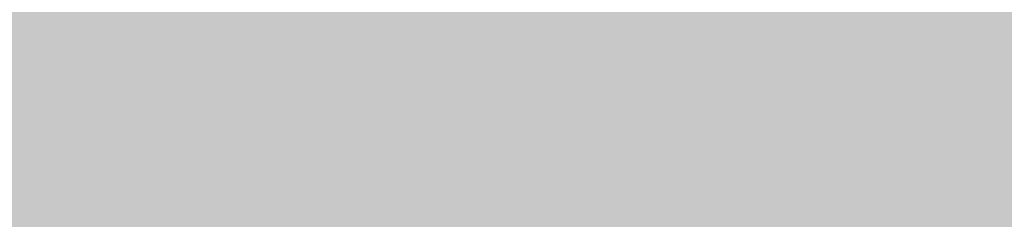
# Model space of a CAD drawing. Units: millimetres. Extents: x 0 to 2267, y 0 to 1823.
# Tile 78 of 256: x 1600.369 to 1605.705, y 1226.115 to 1227.196. Entities that reach past the tile are written whole.
import ezdxf

# ---------------------------------------------------------------- set-up
doc = ezdxf.new("R2010")
doc.units = ezdxf.units.MM
doc.header["$MEASUREMENT"] = 0
doc.layers.add('M-HATC', color=252, linetype='Continuous', lineweight=18)

msp = doc.modelspace()

# ---------------------------------------------------------------- hatches: boundary and pattern name
at = {"layer": 'M-HATC'}
h = msp.add_hatch(color=256, dxfattribs=at)
h.dxf.hatch_style = 1
h.paths.add_polyline_path([(2055.771, 1603.062), (1381.0868, 1603.062), (1381.0868, 1598.062), (2055.771, 1598.062)])
h.paths.add_polyline_path([(2055.771, 1598.062), (1381.0868, 1598.062), (1381.0868, 1593.062), (2055.771, 1593.062)])
h.paths.add_polyline_path([(2051.3074, 1536.7609), (1385.5504, 1536.7609), (1385.5504, 1526.7609), (1387.5504, 1526.7609), (1388.5366, 1525.0528), (1385.3319, 1521.2335), (1385.3319, 1521.2226), (2050.2542, 1522.7491), (2048.3212, 1525.0528), (2049.3074, 1526.7609), (2051.3074, 1526.7609)])
edge = h.paths.add_edge_path()
edge.add_arc((1847.5345, 1379.1492), 135, 222.603061, 222.890851, ccw=False)
edge.add_line((1748.1663, 1287.7656), (1683.0921, 1287.7656))
edge.add_arc((1583.7239, 1379.1492), 135, 317.109149, 317.396939, ccw=False)
edge.add_arc((1678.9686, 1290.6707), 5, 222.8909, 317.1091, ccw=False)
edge.add_arc((1774.2133, 1379.1492), 135, 222.603061, 222.890851, ccw=False)
edge.add_line((1674.8451, 1287.7656), (1609.7709, 1287.7656))
edge.add_arc((1510.4027, 1379.1492), 135, 317.109149, 317.396939, ccw=False)
edge.add_arc((1605.6474, 1290.6707), 5, 222.8909, 317.1091, ccw=False)
edge.add_arc((1700.8921, 1379.1492), 135, 222.603061, 222.890851, ccw=False)
edge.add_line((1601.5239, 1287.7656), (1536.4497, 1287.7656))
edge.add_arc((1437.0815, 1379.1492), 135, 317.109149, 317.396939, ccw=False)
edge.add_arc((1532.3262, 1290.6707), 5, 222.8909, 317.1091, ccw=False)
edge.add_arc((1627.5709, 1379.1492), 135, 222.603061, 222.890851, ccw=False)
edge.add_line((1528.2027, 1287.7656), (1505.9289, 1287.7656))
edge.add_spline(control_points=[(1505.9289, 1287.7656), (1504.2622, 1287.7656), (1504.2622, 1282.7656), (1505.9289, 1282.7656)], knot_values=[0, 0, 0, 0, 5, 5, 5, 5], degree=3, periodic=0)
edge.add_line((1505.9289, 1282.7656), (1930.9289, 1282.7656))
edge.add_spline(control_points=[(1930.9289, 1282.7656), (1932.5956, 1282.7656), (1932.5956, 1287.7656), (1930.9289, 1287.7656)], knot_values=[0, 0, 0, 0, 5, 5, 5, 5], degree=3, periodic=0)
edge.add_line((1930.9289, 1287.7656), (1903.0557, 1287.7656))
edge.add_arc((1803.6875, 1379.1492), 135, 317.109149, 317.396939, ccw=False)
edge.add_arc((1898.9322, 1290.6707), 5, 222.8909, 317.1091, ccw=False)
edge.add_arc((1994.1769, 1379.1492), 135, 222.603061, 222.890851, ccw=False)
edge.add_line((1894.8087, 1287.7656), (1829.7345, 1287.7656))
edge.add_arc((1730.3663, 1379.1492), 135, 317.109149, 317.396939, ccw=False)
edge.add_arc((1825.611, 1290.6707), 5, 222.8909, 317.1091, ccw=False)
edge.add_arc((1920.8557, 1379.1492), 135, 222.603061, 222.890851, ccw=False)
edge.add_line((1821.4875, 1287.7656), (1756.4133, 1287.7656))
edge.add_arc((1657.0451, 1379.1492), 135, 317.109149, 317.396939, ccw=False)
edge.add_arc((1752.2898, 1290.6707), 5, 222.8909, 317.1091, ccw=False)
edge = h.paths.add_edge_path()
edge.add_spline(control_points=[(1843.4289, 1227.2475), (1845.0956, 1227.2475), (1845.0956, 1232.2475), (1843.4289, 1232.2475)], knot_values=[0, 0, 0, 0, 5, 5, 5, 5], degree=3, periodic=0)
edge.add_line((1843.4289, 1232.2475), (1593.4289, 1232.2475))
edge.add_spline(control_points=[(1593.4289, 1232.2475), (1591.7622, 1232.2475), (1591.7622, 1227.2475), (1593.4289, 1227.2475)], knot_values=[0, 0, 0, 0, 5, 5, 5, 5], degree=3, periodic=0)
edge.add_line((1593.4289, 1227.2475), (1843.4289, 1227.2475))
h.paths.add_polyline_path([(1905.9289, 1127.4171), (1530.9289, 1127.4171, 0.414214), (1520.9289, 1117.4171), (1530.9289, 1117.4171), (1915.9289, 1117.4171, 0.414214)])
edge = h.paths.add_edge_path()
edge.add_arc((1397.0858, 1498.4078), 12.7299, 90.78215, 190.87871, ccw=False)
edge.add_line((1396.912, 1511.1365), (1428.0097, 1511.3488))
edge.add_line((1428.0097, 1511.3488), (1433.0097, 1511.3488))
edge.add_line((1433.0097, 1511.3488), (1434.439, 1511.3488))
edge.add_arc((1419.474, 1498.0804), 20, 41.561, 74.08211)
edge.add_line((1424.9592, 1517.3135), (1399.9351, 1517.2561))
edge.add_spline(control_points=[(1399.9307, 1517.2561), (1399.884, 1517.2131), (1399.8328, 1517.1689), (1399.7774, 1517.1236)], knot_values=[11.567499, 11.567499, 11.567499, 11.567499, 11.814249, 11.814249, 11.814249, 11.814249], degree=3, periodic=0)
edge.add_spline(control_points=[(1399.6328, 1517.0099), (1399.5831, 1516.9721), (1399.5307, 1516.9338), (1399.4759, 1516.8947)], knot_values=[11.167718, 11.167718, 11.167718, 11.167718, 11.365188, 11.365188, 11.365188, 11.365188], degree=3, periodic=0)
edge.add_spline(control_points=[(1399.3398, 1516.8001), (1399.1514, 1516.6719), (1398.9384, 1516.5377), (1398.704, 1516.3994)], knot_values=[10.376405, 10.376405, 10.376405, 10.376405, 11.00994, 11.00994, 11.00994, 11.00994], degree=3, periodic=0)
edge.add_spline(control_points=[(1398.6572, 1516.3719), (1398.5789, 1516.326), (1398.4983, 1516.2797), (1398.4155, 1516.2331)], knot_values=[10.125175, 10.125175, 10.125175, 10.125175, 10.334406, 10.334406, 10.334406, 10.334406], degree=3, periodic=0)
edge.add_spline(control_points=[(1398.2642, 1516.1487), (1398.196, 1516.1111), (1398.1263, 1516.0732), (1398.0555, 1516.0351)], knot_values=[9.832246, 9.832246, 9.832246, 9.832246, 9.999658, 9.999658, 9.999658, 9.999658], degree=3, periodic=0)
edge.add_spline(control_points=[(1397.9987, 1516.0048), (1397.7312, 1515.8621), (1397.446, 1515.7171), (1397.1466, 1515.5714)], knot_values=[9.161808, 9.161808, 9.161808, 9.161808, 9.787769, 9.787769, 9.787769, 9.787769], degree=3, periodic=0)
edge.add_spline(control_points=[(1397.1466, 1515.5714), (1396.8418, 1515.423), (1396.5222, 1515.274), (1396.1914, 1515.1262)], knot_values=[8.524455, 8.524455, 8.524455, 8.524455, 9.161808, 9.161808, 9.161808, 9.161808], degree=3, periodic=0)
edge.add_spline(control_points=[(1396.0777, 1515.0756), (1395.9854, 1515.0348), (1395.8922, 1514.994), (1395.7983, 1514.9534)], knot_values=[8.275193, 8.275193, 8.275193, 8.275193, 8.451726, 8.451726, 8.451726, 8.451726], degree=3, periodic=0)
edge.add_spline(control_points=[(1395.6018, 1514.8691), (1395.4997, 1514.8257), (1395.3968, 1514.7824), (1395.2932, 1514.7394)], knot_values=[7.962917, 7.962917, 7.962917, 7.962917, 8.152764, 8.152764, 8.152764, 8.152764], degree=3, periodic=0)
edge.add_spline(control_points=[(1395.2116, 1514.7057), (1394.8278, 1514.5475), (1394.4345, 1514.3929), (1394.0364, 1514.2442)], knot_values=[7.21254, 7.21254, 7.21254, 7.21254, 7.913148, 7.913148, 7.913148, 7.913148], degree=3, periodic=0)
edge.add_spline(control_points=[(1394.0364, 1514.2442), (1393.7076, 1514.1214), (1393.3754, 1514.0027), (1393.0427, 1513.8895)], knot_values=[6.633733, 6.633733, 6.633733, 6.633733, 7.21254, 7.21254, 7.21254, 7.21254], degree=3, periodic=0)
edge.add_spline(control_points=[(1392.8214, 1513.815), (1392.7198, 1513.7812), (1392.6181, 1513.7479), (1392.5166, 1513.7152)], knot_values=[6.328796, 6.328796, 6.328796, 6.328796, 6.505493, 6.505493, 6.505493, 6.505493], degree=3, periodic=0)
edge.add_spline(control_points=[(1392.5166, 1513.7152), (1392.3187, 1513.6515), (1392.1212, 1513.59), (1391.9244, 1513.531)], knot_values=[5.984605, 5.984605, 5.984605, 5.984605, 6.328796, 6.328796, 6.328796, 6.328796], degree=3, periodic=0)
edge.add_spline(control_points=[(1391.7915, 1513.4915), (1391.3122, 1513.3501), (1390.8384, 1513.2239), (1390.3784, 1513.1171)], knot_values=[5.066697, 5.066697, 5.066697, 5.066697, 5.907055, 5.907055, 5.907055, 5.907055], degree=3, periodic=0)
edge.add_spline(control_points=[(1390.3784, 1513.1171), (1390.1797, 1513.071), (1389.9836, 1513.0284), (1389.7907, 1512.9899)], knot_values=[4.70367, 4.70367, 4.70367, 4.70367, 5.066695, 5.066695, 5.066695, 5.066695], degree=3, periodic=0)
edge.add_spline(control_points=[(1389.422, 1512.9204), (1389.2459, 1512.8892), (1389.0729, 1512.8617), (1388.9036, 1512.8381)], knot_values=[4.130571, 4.130571, 4.130571, 4.130571, 4.469816, 4.469816, 4.469816, 4.469816], degree=3, periodic=0)
edge.add_spline(control_points=[(1388.9036, 1512.8381), (1388.591, 1512.7946), (1388.2911, 1512.7644), (1388.0071, 1512.7494)], knot_values=[3.504031, 3.504031, 3.504031, 3.504031, 4.130571, 4.130571, 4.130571, 4.130571], degree=3, periodic=0)
edge.add_spline(control_points=[(1387.9356, 1512.7459), (1387.8538, 1512.7423), (1387.7733, 1512.74), (1387.6944, 1512.739)], knot_values=[3.268866, 3.268866, 3.268866, 3.268866, 3.451164, 3.451164, 3.451164, 3.451164], degree=3, periodic=0)
edge.add_spline(control_points=[(1387.3351, 1512.7443), (1387.2076, 1512.7499), (1387.0847, 1512.7597), (1386.967, 1512.7739)], knot_values=[2.670686, 2.670686, 2.670686, 2.670686, 2.984, 2.984, 2.984, 2.984], degree=3, periodic=0)
edge.add_spline(control_points=[(1386.8327, 1512.7922), (1386.8209, 1512.7941), (1386.8092, 1512.7959), (1386.7975, 1512.7979)], knot_values=[2.516981, 2.516981, 2.516981, 2.516981, 2.549528, 2.549528, 2.549528, 2.549528], degree=3, periodic=0)
edge.add_spline(control_points=[(1386.4526, 1512.8735), (1386.4257, 1512.881), (1386.3993, 1512.889), (1386.3733, 1512.8972)], knot_values=[2.095869, 2.095869, 2.095869, 2.095869, 2.17941, 2.17941, 2.17941, 2.17941], degree=3, periodic=0)
edge.add_spline(control_points=[(1386.0691, 1513.0189), (1386.0634, 1513.0217), (1386.0577, 1513.0246), (1386.052, 1513.0275)], knot_values=[1.72453, 1.72453, 1.72453, 1.72453, 1.745933, 1.745933, 1.745933, 1.745933], degree=3, periodic=0)
edge.add_arc((1399.474, 1498.0804), 20, 131.82432, 180)
edge.add_arc((1630.3336, 1505.5484), 250.9708, 181.705176, 236.427975)
edge.add_arc((1605.3399, 1483.3044), 218.7822, 238.660829, 243.34961)
edge.add_arc((1647.0911, 1510.3592), 262.8986, 183.129836, 237.853442, ccw=False)
h.paths.add_polyline_path([(1406.5369, 1391.9644, 0.149382), (1491.5506, 1296.4418, -0.129517)], flags=17)
edge = h.paths.add_edge_path()
edge.add_arc((2037.3838, 1498.0804), 20, 0, 48.26587)
edge.add_spline(control_points=[(2050.6973, 1513.0052), (2050.6512, 1512.9847), (2050.6034, 1512.9655), (2050.5539, 1512.9477)], knot_values=[1.835652, 1.835652, 1.835652, 1.835652, 2.000781, 2.000781, 2.000781, 2.000781], degree=3, periodic=0)
edge.add_spline(control_points=[(2050.4616, 1512.9166), (2050.479, 1512.9221), (2050.4963, 1512.9277), (2050.5133, 1512.9335)], knot_values=[2.045477, 2.045477, 2.045477, 2.045477, 2.101389, 2.101389, 2.101389, 2.101389], degree=3, periodic=0)
edge.add_spline(control_points=[(2050.129, 1512.8342), (2050.1984, 1512.8473), (2050.2657, 1512.8623), (2050.3308, 1512.8792)], knot_values=[2.237629, 2.237629, 2.237629, 2.237629, 2.435841, 2.435841, 2.435841, 2.435841], degree=3, periodic=0)
edge.add_spline(control_points=[(2050.0946, 1512.8278), (2050.1061, 1512.8299), (2050.1176, 1512.832), (2050.129, 1512.8342)], knot_values=[2.435841, 2.435841, 2.435841, 2.435841, 2.468321, 2.468321, 2.468321, 2.468321], degree=3, periodic=0)
edge.add_spline(control_points=[(2049.7843, 1512.7851), (2049.8552, 1512.7922), (2049.9243, 1512.8008), (2049.9917, 1512.8109)], knot_values=[2.563852, 2.563852, 2.563852, 2.563852, 2.748541, 2.748541, 2.748541, 2.748541], degree=3, periodic=0)
edge.add_spline(control_points=[(2049.4052, 1512.7617), (2049.5364, 1512.7653), (2049.6629, 1512.773), (2049.7843, 1512.7851)], knot_values=[2.748541, 2.748541, 2.748541, 2.748541, 3.064882, 3.064882, 3.064882, 3.064882], degree=3, periodic=0)
edge.add_spline(control_points=[(2049.1698, 1512.7597), (2049.2336, 1512.7591), (2049.2965, 1512.7594), (2049.3584, 1512.7606)], knot_values=[3.102309, 3.102309, 3.102309, 3.102309, 3.2503, 3.2503, 3.2503, 3.2503], degree=3, periodic=0)
edge.add_spline(control_points=[(2048.8573, 1512.7691), (2048.9638, 1512.7638), (2049.068, 1512.7606), (2049.1698, 1512.7597)], knot_values=[3.2503, 3.2503, 3.2503, 3.2503, 3.486069, 3.486069, 3.486069, 3.486069], degree=3, periodic=0)
edge.add_spline(control_points=[(2048.6924, 1512.7789), (2048.3729, 1512.8009), (2048.0345, 1512.8411), (2047.6817, 1512.897)], knot_values=[3.606429, 3.606429, 3.606429, 3.606429, 4.2989, 4.2989, 4.2989, 4.2989], degree=3, periodic=0)
edge.add_spline(control_points=[(2047.6817, 1512.897), (2047.5458, 1512.9185), (2047.4077, 1512.9424), (2047.2678, 1512.9685)], knot_values=[4.2989, 4.2989, 4.2989, 4.2989, 4.565769, 4.565769, 4.565769, 4.565769], degree=3, periodic=0)
edge.add_spline(control_points=[(2047.2678, 1512.9685), (2047.1449, 1512.9914), (2047.0207, 1513.016), (2046.8951, 1513.0422)], knot_values=[4.565769, 4.565769, 4.565769, 4.565769, 4.799971, 4.799971, 4.799971, 4.799971], degree=3, periodic=0)
edge.add_spline(control_points=[(2046.8951, 1513.0422), (2046.5286, 1513.1188), (2046.1513, 1513.209), (2045.7676, 1513.3107)], knot_values=[4.799971, 4.799971, 4.799971, 4.799971, 5.483718, 5.483718, 5.483718, 5.483718], degree=3, periodic=0)
edge.add_spline(control_points=[(2045.7676, 1513.3107), (2045.3724, 1513.4154), (2044.9704, 1513.5322), (2044.5662, 1513.6588)], knot_values=[5.483718, 5.483718, 5.483718, 5.483718, 6.187866, 6.187866, 6.187866, 6.187866], degree=3, periodic=0)
edge.add_spline(control_points=[(2044.5662, 1513.6588), (2044.4149, 1513.7061), (2044.2633, 1513.7549), (2044.1116, 1513.8048)], knot_values=[6.187866, 6.187866, 6.187866, 6.187866, 6.451551, 6.451551, 6.451551, 6.451551], degree=3, periodic=0)
edge.add_spline(control_points=[(2044.1116, 1513.8048), (2043.9967, 1513.8427), (2043.8817, 1513.8813), (2043.7668, 1513.9205)], knot_values=[6.451551, 6.451551, 6.451551, 6.451551, 6.651434, 6.651434, 6.651434, 6.651434], degree=3, periodic=0)
edge.add_spline(control_points=[(2043.7668, 1513.9205), (2043.3716, 1514.0554), (2042.9774, 1514.1979), (2042.5886, 1514.3458)], knot_values=[6.651434, 6.651434, 6.651434, 6.651434, 7.338879, 7.338879, 7.338879, 7.338879], degree=3, periodic=0)
edge.add_spline(control_points=[(2042.5886, 1514.3458), (2042.1643, 1514.5071), (2041.7465, 1514.6749), (2041.3409, 1514.846)], knot_values=[7.338879, 7.338879, 7.338879, 7.338879, 8.089209, 8.089209, 8.089209, 8.089209], degree=3, periodic=0)
edge.add_spline(control_points=[(2041.3409, 1514.846), (2041.1028, 1514.9465), (2040.869, 1515.0481), (2040.6405, 1515.1502)], knot_values=[8.089209, 8.089209, 8.089209, 8.089209, 8.529587, 8.529587, 8.529587, 8.529587], degree=3, periodic=0)
edge.add_spline(control_points=[(2040.51, 1515.2089), (2040.0824, 1515.4022), (2039.6747, 1515.5971), (2039.295, 1515.7894)], knot_values=[8.613818, 8.613818, 8.613818, 8.613818, 9.44571, 9.44571, 9.44571, 9.44571], degree=3, periodic=0)
edge.add_spline(control_points=[(2039.295, 1515.7894), (2039.0618, 1515.9075), (2038.8391, 1516.0246), (2038.6288, 1516.1398)], knot_values=[9.44571, 9.44571, 9.44571, 9.44571, 9.956404, 9.956404, 9.956404, 9.956404], degree=3, periodic=0)
edge.add_spline(control_points=[(2038.6288, 1516.1398), (2038.5187, 1516.2001), (2038.4121, 1516.2598), (2038.309, 1516.3189)], knot_values=[9.956404, 9.956404, 9.956404, 9.956404, 10.223542, 10.223542, 10.223542, 10.223542], degree=3, periodic=0)
edge.add_spline(control_points=[(2038.309, 1516.3189), (2038.2138, 1516.3735), (2038.1216, 1516.4276), (2038.0328, 1516.481)], knot_values=[10.223542, 10.223542, 10.223542, 10.223542, 10.47051, 10.47051, 10.47051, 10.47051], degree=3, periodic=0)
edge.add_spline(control_points=[(2038.0328, 1516.481), (2037.7855, 1516.6296), (2037.5639, 1516.773), (2037.3722, 1516.909)], knot_values=[10.47051, 10.47051, 10.47051, 10.47051, 11.15767, 11.15767, 11.15767, 11.15767], degree=3, periodic=0)
edge.add_spline(control_points=[(2037.3722, 1516.909), (2037.2789, 1516.9752), (2037.1927, 1517.0396), (2037.1142, 1517.102)], knot_values=[11.15767, 11.15767, 11.15767, 11.15767, 11.49227, 11.49227, 11.49227, 11.49227], degree=3, periodic=0)
edge.add_spline(control_points=[(2036.8564, 1517.3259), (2036.9148, 1517.2692), (2036.9814, 1517.2103), (2037.0557, 1517.1492)], knot_values=[11.577341, 11.577341, 11.577341, 11.577341, 11.91035, 11.91035, 11.91035, 11.91035], degree=3, periodic=0)
edge.add_spline(control_points=[(2036.8074, 1517.3748), (2036.823, 1517.3587), (2036.8393, 1517.3424), (2036.8564, 1517.3259)], knot_values=[11.91035, 11.91035, 11.91035, 11.91035, 12.007402, 12.007402, 12.007402, 12.007402], degree=3, periodic=0)
edge.add_spline(control_points=[(2036.7017, 1517.494), (2036.7104, 1517.483), (2036.7196, 1517.4719), (2036.7291, 1517.4606)], knot_values=[12.184155, 12.184155, 12.184155, 12.184155, 12.255409, 12.255409, 12.255409, 12.255409], degree=3, periodic=0)
edge.add_spline(control_points=[(2036.6159, 1517.6205), (2036.62, 1517.613), (2036.6243, 1517.6055), (2036.6289, 1517.5979)], knot_values=[12.487913, 12.487913, 12.487913, 12.487913, 12.541035, 12.541035, 12.541035, 12.541035], degree=3, periodic=0)
edge.add_spline(control_points=[(2036.5635, 1517.786), (2036.5637, 1517.7794), (2036.5642, 1517.7726), (2036.565, 1517.7658)], knot_values=[12.911761, 12.911761, 12.911761, 12.911761, 12.968286, 12.968286, 12.968286, 12.968286], degree=3, periodic=0)
edge.add_spline(control_points=[(2036.6166, 1517.9304), (2036.6125, 1517.9259), (2036.6086, 1517.9212), (2036.6049, 1517.9165)], knot_values=[13.382527, 13.382527, 13.382527, 13.382527, 13.433791, 13.433791, 13.433791, 13.433791], degree=3, periodic=0)
edge.add_spline(control_points=[(2036.749, 1518.017), (2036.7361, 1518.0116), (2036.7239, 1518.006), (2036.7124, 1518.0002)], knot_values=[13.726299, 13.726299, 13.726299, 13.726299, 13.809928, 13.809928, 13.809928, 13.809928], degree=3, periodic=0)
edge.add_spline(control_points=[(2036.8604, 1518.0528), (2036.8386, 1518.0474), (2036.8181, 1518.0416), (2036.7988, 1518.0353)], knot_values=[13.910887, 13.910887, 13.910887, 13.910887, 14.02153, 14.02153, 14.02153, 14.02153], degree=3, periodic=0)
edge.add_line((2036.9639, 1518.0804), (2032.3838, 1518.0804))
edge.add_line((2032.3838, 1518.0804), (2027.3838, 1518.0804))
edge.add_line((2027.3838, 1518.0804), (2022.3838, 1518.0804))
edge.add_line((2022.3838, 1518.0804), (2017.3838, 1518.0804))
edge.add_arc((2017.3838, 1498.0804), 20, 90, 138.439)
edge.add_line((2002.4188, 1511.3488), (2003.8481, 1511.3488))
edge.add_line((2003.8481, 1511.3488), (2008.8481, 1511.3488))
edge.add_line((2008.8481, 1511.3488), (2039.772, 1511.1377))
edge.add_arc((2039.772, 1498.4078), 12.7299, -10.87871, 90, ccw=False)
edge.add_arc((1789.7668, 1510.3592), 262.8986, 302.146558, 356.870164, ccw=False)
edge.add_arc((1831.5179, 1483.3044), 218.7822, 296.65039, 301.339171)
edge.add_arc((1806.5242, 1505.5484), 250.9708, 303.572025, 358.294824)
h.paths.add_polyline_path([(2030.321, 1391.9644, -0.129517), (1945.3072, 1296.4418, 0.149382)], flags=17)
edge = h.paths.add_edge_path()
edge.add_spline(control_points=[(2037.2464, 1518.0821), (2037.2898, 1518.081), (2037.3355, 1518.0804), (2037.3838, 1518.0804)], knot_values=[0.000012, 0.000012, 0.000012, 0.000012, 0.144754, 0.144754, 0.144754, 0.144754], degree=3, periodic=0)
edge.add_line((2037.3357, 1518.0804), (2037.0096, 1518.0804))
edge.add_spline(control_points=[(2037.0096, 1518.0804), (2036.9822, 1518.0768), (2036.956, 1518.0727), (2036.9312, 1518.0681)], knot_values=[14.13465, 14.13465, 14.13465, 14.13465, 14.247197, 14.247197, 14.247197, 14.247197], degree=3, periodic=0)
edge.add_spline(control_points=[(2036.9312, 1518.0681), (2036.9276, 1518.0674), (2036.9241, 1518.0667), (2036.9205, 1518.0661)], knot_values=[14.118315, 14.118315, 14.118315, 14.118315, 14.13465, 14.13465, 14.13465, 14.13465], degree=3, periodic=0)
edge.add_spline(control_points=[(2036.9205, 1518.0661), (2036.9118, 1518.0644), (2036.9032, 1518.0626), (2036.8948, 1518.0608)], knot_values=[14.078086, 14.078086, 14.078086, 14.078086, 14.118315, 14.118315, 14.118315, 14.118315], degree=3, periodic=0)
edge.add_spline(control_points=[(2036.8948, 1518.0608), (2036.883, 1518.0583), (2036.8716, 1518.0556), (2036.8604, 1518.0528)], knot_values=[14.02153, 14.02153, 14.02153, 14.02153, 14.078086, 14.078086, 14.078086, 14.078086], degree=3, periodic=0)
edge.add_spline(control_points=[(2036.8604, 1518.0528), (2036.8386, 1518.0474), (2036.8181, 1518.0416), (2036.7988, 1518.0353)], knot_values=[13.910887, 13.910887, 13.910887, 13.910887, 14.02153, 14.02153, 14.02153, 14.02153], degree=3, periodic=0)
edge.add_spline(control_points=[(2036.7988, 1518.0353), (2036.7981, 1518.035), (2036.7974, 1518.0348), (2036.7967, 1518.0346)], knot_values=[13.906906, 13.906906, 13.906906, 13.906906, 13.910887, 13.910887, 13.910887, 13.910887], degree=3, periodic=0)
edge.add_spline(control_points=[(2036.7967, 1518.0346), (2036.7882, 1518.0318), (2036.7799, 1518.0289), (2036.7719, 1518.0259)], knot_values=[13.857826, 13.857826, 13.857826, 13.857826, 13.906906, 13.906906, 13.906906, 13.906906], degree=3, periodic=0)
edge.add_spline(control_points=[(2036.7719, 1518.0259), (2036.764, 1518.023), (2036.7564, 1518.02), (2036.749, 1518.017)], knot_values=[13.809928, 13.809928, 13.809928, 13.809928, 13.857826, 13.857826, 13.857826, 13.857826], degree=3, periodic=0)
edge.add_spline(control_points=[(2036.749, 1518.017), (2036.7361, 1518.0116), (2036.7239, 1518.006), (2036.7124, 1518.0002)], knot_values=[13.726299, 13.726299, 13.726299, 13.726299, 13.809928, 13.809928, 13.809928, 13.809928], degree=3, periodic=0)
edge.add_spline(control_points=[(2036.7124, 1518.0002), (2036.7121, 1518), (2036.7118, 1517.9999), (2036.7115, 1517.9997)], knot_values=[13.723993, 13.723993, 13.723993, 13.723993, 13.726299, 13.726299, 13.726299, 13.726299], degree=3, periodic=0)
edge.add_spline(control_points=[(2036.7115, 1517.9997), (2036.7063, 1517.9971), (2036.7013, 1517.9944), (2036.6965, 1517.9917)], knot_values=[13.686536, 13.686536, 13.686536, 13.686536, 13.723993, 13.723993, 13.723993, 13.723993], degree=3, periodic=0)
edge.add_spline(control_points=[(2036.6965, 1517.9917), (2036.6919, 1517.9891), (2036.6874, 1517.9865), (2036.6831, 1517.9839)], knot_values=[13.651251, 13.651251, 13.651251, 13.651251, 13.686536, 13.686536, 13.686536, 13.686536], degree=3, periodic=0)
edge.add_spline(control_points=[(2036.6831, 1517.9839), (2036.6764, 1517.9798), (2036.67, 1517.9757), (2036.6639, 1517.9714)], knot_values=[13.596804, 13.596804, 13.596804, 13.596804, 13.651251, 13.651251, 13.651251, 13.651251], degree=3, periodic=0)
edge.add_spline(control_points=[(2036.6639, 1517.9714), (2036.6636, 1517.9712), (2036.6633, 1517.9709), (2036.6629, 1517.9707)], knot_values=[13.593956, 13.593956, 13.593956, 13.593956, 13.596804, 13.596804, 13.596804, 13.596804], degree=3, periodic=0)
edge.add_spline(control_points=[(2036.6629, 1517.9707), (2036.6603, 1517.9689), (2036.6577, 1517.967), (2036.6552, 1517.9651)], knot_values=[13.570322, 13.570322, 13.570322, 13.570322, 13.593956, 13.593956, 13.593956, 13.593956], degree=3, periodic=0)
edge.add_spline(control_points=[(2036.6552, 1517.9651), (2036.6525, 1517.9631), (2036.6499, 1517.9611), (2036.6474, 1517.9591)], knot_values=[13.545477, 13.545477, 13.545477, 13.545477, 13.570322, 13.570322, 13.570322, 13.570322], degree=3, periodic=0)
edge.add_spline(control_points=[(2036.6474, 1517.9591), (2036.6472, 1517.9589), (2036.6471, 1517.9588), (2036.6469, 1517.9587)], knot_values=[13.543931, 13.543931, 13.543931, 13.543931, 13.545477, 13.545477, 13.545477, 13.545477], degree=3, periodic=0)
edge.add_spline(control_points=[(2036.6469, 1517.9587), (2036.6412, 1517.9541), (2036.6358, 1517.9494), (2036.6307, 1517.9447)], knot_values=[13.488237, 13.488237, 13.488237, 13.488237, 13.543931, 13.543931, 13.543931, 13.543931], degree=3, periodic=0)
edge.add_spline(control_points=[(2036.6307, 1517.9447), (2036.6282, 1517.9423), (2036.6257, 1517.9399), (2036.6233, 1517.9374)], knot_values=[13.460307, 13.460307, 13.460307, 13.460307, 13.488237, 13.488237, 13.488237, 13.488237], degree=3, periodic=0)
edge.add_spline(control_points=[(2036.6233, 1517.9374), (2036.6215, 1517.9356), (2036.6198, 1517.9338), (2036.6181, 1517.932)], knot_values=[13.439712, 13.439712, 13.439712, 13.439712, 13.460307, 13.460307, 13.460307, 13.460307], degree=3, periodic=0)
edge.add_spline(control_points=[(2036.6181, 1517.932), (2036.6176, 1517.9315), (2036.6171, 1517.9309), (2036.6166, 1517.9304)], knot_values=[13.433791, 13.433791, 13.433791, 13.433791, 13.439712, 13.439712, 13.439712, 13.439712], degree=3, periodic=0)
edge.add_spline(control_points=[(2036.6166, 1517.9304), (2036.6125, 1517.9259), (2036.6086, 1517.9212), (2036.6049, 1517.9165)], knot_values=[13.382527, 13.382527, 13.382527, 13.382527, 13.433791, 13.433791, 13.433791, 13.433791], degree=3, periodic=0)
edge.add_spline(control_points=[(2036.6049, 1517.9165), (2036.6026, 1517.9135), (2036.6004, 1517.9104), (2036.5982, 1517.9074)], knot_values=[13.350017, 13.350017, 13.350017, 13.350017, 13.382527, 13.382527, 13.382527, 13.382527], degree=3, periodic=0)
edge.add_spline(control_points=[(2036.5982, 1517.9074), (2036.5972, 1517.9059), (2036.5962, 1517.9043), (2036.5952, 1517.9028)], knot_values=[13.333922, 13.333922, 13.333922, 13.333922, 13.350017, 13.350017, 13.350017, 13.350017], degree=3, periodic=0)
edge.add_spline(control_points=[(2036.5952, 1517.9028), (2036.5945, 1517.9018), (2036.5939, 1517.9009), (2036.5933, 1517.8999)], knot_values=[13.323828, 13.323828, 13.323828, 13.323828, 13.333922, 13.333922, 13.333922, 13.333922], degree=3, periodic=0)
edge.add_spline(control_points=[(2036.5933, 1517.8999), (2036.5905, 1517.8955), (2036.5879, 1517.8909), (2036.5855, 1517.8864)], knot_values=[13.277545, 13.277545, 13.277545, 13.277545, 13.323828, 13.323828, 13.323828, 13.323828], degree=3, periodic=0)
edge.add_spline(control_points=[(2036.5855, 1517.8864), (2036.5836, 1517.8827), (2036.5817, 1517.8789), (2036.5801, 1517.8751)], knot_values=[13.240119, 13.240119, 13.240119, 13.240119, 13.277545, 13.277545, 13.277545, 13.277545], degree=3, periodic=0)
edge.add_spline(control_points=[(2036.5801, 1517.8751), (2036.5795, 1517.8739), (2036.579, 1517.8727), (2036.5785, 1517.8715)], knot_values=[13.228211, 13.228211, 13.228211, 13.228211, 13.240119, 13.240119, 13.240119, 13.240119], degree=3, periodic=0)
edge.add_spline(control_points=[(2036.5785, 1517.8715), (2036.578, 1517.8702), (2036.5774, 1517.869), (2036.5769, 1517.8677)], knot_values=[13.215717, 13.215717, 13.215717, 13.215717, 13.228211, 13.228211, 13.228211, 13.228211], degree=3, periodic=0)
edge.add_spline(control_points=[(2036.5769, 1517.8677), (2036.5755, 1517.864), (2036.5741, 1517.8603), (2036.5729, 1517.8565)], knot_values=[13.179847, 13.179847, 13.179847, 13.179847, 13.215717, 13.215717, 13.215717, 13.215717], degree=3, periodic=0)
edge.add_spline(control_points=[(2036.5729, 1517.8565), (2036.5713, 1517.8515), (2036.5699, 1517.8464), (2036.5687, 1517.8413)], knot_values=[13.132017, 13.132017, 13.132017, 13.132017, 13.179847, 13.179847, 13.179847, 13.179847], degree=3, periodic=0)
edge.add_spline(control_points=[(2036.5687, 1517.8413), (2036.5684, 1517.8402), (2036.5682, 1517.8392), (2036.568, 1517.8382)], knot_values=[13.122482, 13.122482, 13.122482, 13.122482, 13.132017, 13.132017, 13.132017, 13.132017], degree=3, periodic=0)
edge.add_spline(control_points=[(2036.568, 1517.8382), (2036.5676, 1517.8363), (2036.5672, 1517.8345), (2036.5669, 1517.8327)], knot_values=[13.105592, 13.105592, 13.105592, 13.105592, 13.122482, 13.122482, 13.122482, 13.122482], degree=3, periodic=0)
edge.add_spline(control_points=[(2036.5669, 1517.8327), (2036.5662, 1517.8292), (2036.5657, 1517.8257), (2036.5652, 1517.8222)], knot_values=[13.074063, 13.074063, 13.074063, 13.074063, 13.105592, 13.105592, 13.105592, 13.105592], degree=3, periodic=0)
edge.add_spline(control_points=[(2036.5652, 1517.8222), (2036.5652, 1517.8222), (2036.5652, 1517.8222), (2036.5652, 1517.8222)], knot_values=[13.074043, 13.074043, 13.074043, 13.074043, 13.074063, 13.074063, 13.074063, 13.074063], degree=3, periodic=0)
edge.add_spline(control_points=[(2036.5652, 1517.8222), (2036.5644, 1517.8164), (2036.5639, 1517.8106), (2036.5636, 1517.8046)], knot_values=[13.021884, 13.021884, 13.021884, 13.021884, 13.074043, 13.074043, 13.074043, 13.074043], degree=3, periodic=0)
edge.add_spline(control_points=[(2036.5636, 1517.8046), (2036.5636, 1517.804), (2036.5636, 1517.8034), (2036.5635, 1517.8028)], knot_values=[13.01674, 13.01674, 13.01674, 13.01674, 13.021884, 13.021884, 13.021884, 13.021884], degree=3, periodic=0)
edge.add_spline(control_points=[(2036.5635, 1517.8028), (2036.5634, 1517.8005), (2036.5634, 1517.7982), (2036.5634, 1517.7958)], knot_values=[12.996438, 12.996438, 12.996438, 12.996438, 13.01674, 13.01674, 13.01674, 13.01674], degree=3, periodic=0)
edge.add_spline(control_points=[(2036.5634, 1517.7958), (2036.5633, 1517.7926), (2036.5634, 1517.7893), (2036.5635, 1517.786)], knot_values=[12.968286, 12.968286, 12.968286, 12.968286, 12.996438, 12.996438, 12.996438, 12.996438], degree=3, periodic=0)
edge.add_spline(control_points=[(2036.5635, 1517.786), (2036.5637, 1517.7794), (2036.5642, 1517.7726), (2036.565, 1517.7658)], knot_values=[12.911761, 12.911761, 12.911761, 12.911761, 12.968286, 12.968286, 12.968286, 12.968286], degree=3, periodic=0)
edge.add_spline(control_points=[(2036.565, 1517.7658), (2036.565, 1517.7657), (2036.565, 1517.7656), (2036.565, 1517.7656)], knot_values=[12.911017, 12.911017, 12.911017, 12.911017, 12.911761, 12.911761, 12.911761, 12.911761], degree=3, periodic=0)
edge.add_spline(control_points=[(2036.565, 1517.7656), (2036.5654, 1517.7625), (2036.5658, 1517.7593), (2036.5663, 1517.7562)], knot_values=[12.88528, 12.88528, 12.88528, 12.88528, 12.911017, 12.911017, 12.911017, 12.911017], degree=3, periodic=0)
edge.add_spline(control_points=[(2036.5663, 1517.7562), (2036.5667, 1517.7534), (2036.5672, 1517.7506), (2036.5677, 1517.7478)], knot_values=[12.862519, 12.862519, 12.862519, 12.862519, 12.88528, 12.88528, 12.88528, 12.88528], degree=3, periodic=0)
edge.add_spline(control_points=[(2036.5677, 1517.7478), (2036.5678, 1517.7474), (2036.5679, 1517.7469), (2036.568, 1517.7465)], knot_values=[12.858885, 12.858885, 12.858885, 12.858885, 12.862519, 12.862519, 12.862519, 12.862519], degree=3, periodic=0)
edge.add_spline(control_points=[(2036.568, 1517.7465), (2036.5692, 1517.7399), (2036.5707, 1517.7332), (2036.5724, 1517.7264)], knot_values=[12.8053, 12.8053, 12.8053, 12.8053, 12.858885, 12.858885, 12.858885, 12.858885], degree=3, periodic=0)
edge.add_spline(control_points=[(2036.5724, 1517.7264), (2036.5734, 1517.7226), (2036.5745, 1517.7187), (2036.5756, 1517.7149)], knot_values=[12.775176, 12.775176, 12.775176, 12.775176, 12.8053, 12.8053, 12.8053, 12.8053], degree=3, periodic=0)
edge.add_spline(control_points=[(2036.5756, 1517.7149), (2036.5763, 1517.7125), (2036.577, 1517.7102), (2036.5778, 1517.7078)], knot_values=[12.756759, 12.756759, 12.756759, 12.756759, 12.775176, 12.775176, 12.775176, 12.775176], degree=3, periodic=0)
edge.add_spline(control_points=[(2036.5778, 1517.7078), (2036.5781, 1517.7067), (2036.5784, 1517.7057), (2036.5787, 1517.7047)], knot_values=[12.748742, 12.748742, 12.748742, 12.748742, 12.756759, 12.756759, 12.756759, 12.756759], degree=3, periodic=0)
edge.add_spline(control_points=[(2036.5787, 1517.7047), (2036.5808, 1517.6983), (2036.5831, 1517.6919), (2036.5856, 1517.6854)], knot_values=[12.69959, 12.69959, 12.69959, 12.69959, 12.748742, 12.748742, 12.748742, 12.748742], degree=3, periodic=0)
edge.add_spline(control_points=[(2036.5856, 1517.6854), (2036.5876, 1517.68), (2036.5898, 1517.6746), (2036.5921, 1517.6692)], knot_values=[12.659038, 12.659038, 12.659038, 12.659038, 12.69959, 12.69959, 12.69959, 12.69959], degree=3, periodic=0)
edge.add_spline(control_points=[(2036.5921, 1517.6692), (2036.594, 1517.6648), (2036.5959, 1517.6605), (2036.5979, 1517.6561)], knot_values=[12.626806, 12.626806, 12.626806, 12.626806, 12.659038, 12.659038, 12.659038, 12.659038], degree=3, periodic=0)
edge.add_spline(control_points=[(2036.5979, 1517.6561), (2036.5984, 1517.6551), (2036.5989, 1517.6541), (2036.5993, 1517.6531)], knot_values=[12.619394, 12.619394, 12.619394, 12.619394, 12.626806, 12.626806, 12.626806, 12.626806], degree=3, periodic=0)
edge.add_spline(control_points=[(2036.5993, 1517.6531), (2036.6043, 1517.6424), (2036.6099, 1517.6315), (2036.6159, 1517.6205)], knot_values=[12.541039, 12.541039, 12.541039, 12.541039, 12.619394, 12.619394, 12.619394, 12.619394], degree=3, periodic=0)
edge.add_spline(control_points=[(2036.6159, 1517.6205), (2036.6159, 1517.6205), (2036.6159, 1517.6205), (2036.6159, 1517.6205)], knot_values=[12.541035, 12.541035, 12.541035, 12.541035, 12.541039, 12.541039, 12.541039, 12.541039], degree=3, periodic=0)
edge.add_spline(control_points=[(2036.6159, 1517.6205), (2036.62, 1517.613), (2036.6243, 1517.6055), (2036.6289, 1517.5979)], knot_values=[12.487913, 12.487913, 12.487913, 12.487913, 12.541035, 12.541035, 12.541035, 12.541035], degree=3, periodic=0)
edge.add_spline(control_points=[(2036.6289, 1517.5979), (2036.6326, 1517.5916), (2036.6365, 1517.5853), (2036.6406, 1517.5789)], knot_values=[12.443982, 12.443982, 12.443982, 12.443982, 12.487913, 12.487913, 12.487913, 12.487913], degree=3, periodic=0)
edge.add_spline(control_points=[(2036.6406, 1517.5789), (2036.6414, 1517.5776), (2036.6423, 1517.5763), (2036.6431, 1517.5749)], knot_values=[12.434996, 12.434996, 12.434996, 12.434996, 12.443982, 12.443982, 12.443982, 12.443982], degree=3, periodic=0)
edge.add_spline(control_points=[(2036.6431, 1517.5749), (2036.6531, 1517.5596), (2036.6639, 1517.5439), (2036.6756, 1517.528)], knot_values=[12.329647, 12.329647, 12.329647, 12.329647, 12.434996, 12.434996, 12.434996, 12.434996], degree=3, periodic=0)
edge.add_spline(control_points=[(2036.6756, 1517.528), (2036.6839, 1517.5168), (2036.6925, 1517.5055), (2036.7017, 1517.494)], knot_values=[12.255409, 12.255409, 12.255409, 12.255409, 12.329647, 12.329647, 12.329647, 12.329647], degree=3, periodic=0)
edge.add_spline(control_points=[(2036.7017, 1517.494), (2036.7104, 1517.483), (2036.7196, 1517.4719), (2036.7291, 1517.4606)], knot_values=[12.184155, 12.184155, 12.184155, 12.184155, 12.255409, 12.255409, 12.255409, 12.255409], degree=3, periodic=0)
edge.add_spline(control_points=[(2036.7291, 1517.4606), (2036.7436, 1517.4435), (2036.759, 1517.4262), (2036.7753, 1517.4085)], knot_values=[12.075961, 12.075961, 12.075961, 12.075961, 12.184155, 12.184155, 12.184155, 12.184155], degree=3, periodic=0)
edge.add_spline(control_points=[(2036.7753, 1517.4085), (2036.7763, 1517.4075), (2036.7773, 1517.4064), (2036.7783, 1517.4054)], knot_values=[12.069502, 12.069502, 12.069502, 12.069502, 12.075961, 12.075961, 12.075961, 12.075961], degree=3, periodic=0)
edge.add_spline(control_points=[(2036.7783, 1517.4054), (2036.7877, 1517.3953), (2036.7974, 1517.385), (2036.8074, 1517.3748)], knot_values=[12.007402, 12.007402, 12.007402, 12.007402, 12.069502, 12.069502, 12.069502, 12.069502], degree=3, periodic=0)
edge.add_spline(control_points=[(2036.8074, 1517.3748), (2036.823, 1517.3587), (2036.8393, 1517.3424), (2036.8564, 1517.3259)], knot_values=[11.91035, 11.91035, 11.91035, 11.91035, 12.007402, 12.007402, 12.007402, 12.007402], degree=3, periodic=0)
edge.add_spline(control_points=[(2036.8564, 1517.3259), (2036.9148, 1517.2692), (2036.9814, 1517.2103), (2037.0557, 1517.1492)], knot_values=[11.577341, 11.577341, 11.577341, 11.577341, 11.91035, 11.91035, 11.91035, 11.91035], degree=3, periodic=0)
edge.add_spline(control_points=[(2037.0557, 1517.1492), (2037.0747, 1517.1336), (2037.0942, 1517.1179), (2037.1142, 1517.102)], knot_values=[11.49227, 11.49227, 11.49227, 11.49227, 11.577341, 11.577341, 11.577341, 11.577341], degree=3, periodic=0)
edge.add_spline(control_points=[(2037.1142, 1517.102), (2037.1927, 1517.0396), (2037.2789, 1516.9752), (2037.3722, 1516.909)], knot_values=[11.15767, 11.15767, 11.15767, 11.15767, 11.49227, 11.49227, 11.49227, 11.49227], degree=3, periodic=0)
edge.add_spline(control_points=[(2037.3722, 1516.909), (2037.5639, 1516.773), (2037.7855, 1516.6296), (2038.0328, 1516.481)], knot_values=[10.47051, 10.47051, 10.47051, 10.47051, 11.15767, 11.15767, 11.15767, 11.15767], degree=3, periodic=0)
edge.add_spline(control_points=[(2038.0328, 1516.481), (2038.1216, 1516.4276), (2038.2138, 1516.3735), (2038.309, 1516.3189)], knot_values=[10.223542, 10.223542, 10.223542, 10.223542, 10.47051, 10.47051, 10.47051, 10.47051], degree=3, periodic=0)
edge.add_spline(control_points=[(2038.309, 1516.3189), (2038.4121, 1516.2598), (2038.5187, 1516.2001), (2038.6288, 1516.1398)], knot_values=[9.956404, 9.956404, 9.956404, 9.956404, 10.223542, 10.223542, 10.223542, 10.223542], degree=3, periodic=0)
edge.add_spline(control_points=[(2038.6288, 1516.1398), (2038.8391, 1516.0246), (2039.0618, 1515.9075), (2039.295, 1515.7894)], knot_values=[9.44571, 9.44571, 9.44571, 9.44571, 9.956404, 9.956404, 9.956404, 9.956404], degree=3, periodic=0)
edge.add_spline(control_points=[(2039.295, 1515.7894), (2039.6747, 1515.5971), (2040.0824, 1515.4022), (2040.51, 1515.2089)], knot_values=[8.613818, 8.613818, 8.613818, 8.613818, 9.44571, 9.44571, 9.44571, 9.44571], degree=3, periodic=0)
edge.add_spline(control_points=[(2040.51, 1515.2089), (2040.5533, 1515.1893), (2040.5968, 1515.1697), (2040.6405, 1515.1502)], knot_values=[8.529587, 8.529587, 8.529587, 8.529587, 8.613818, 8.613818, 8.613818, 8.613818], degree=3, periodic=0)
edge.add_spline(control_points=[(2040.6405, 1515.1502), (2040.869, 1515.0481), (2041.1028, 1514.9465), (2041.3409, 1514.846)], knot_values=[8.089209, 8.089209, 8.089209, 8.089209, 8.529587, 8.529587, 8.529587, 8.529587], degree=3, periodic=0)
edge.add_spline(control_points=[(2041.3409, 1514.846), (2041.7465, 1514.6749), (2042.1643, 1514.5071), (2042.5886, 1514.3458)], knot_values=[7.338879, 7.338879, 7.338879, 7.338879, 8.089209, 8.089209, 8.089209, 8.089209], degree=3, periodic=0)
edge.add_spline(control_points=[(2042.5886, 1514.3458), (2042.9774, 1514.1979), (2043.3716, 1514.0554), (2043.7668, 1513.9205)], knot_values=[6.651434, 6.651434, 6.651434, 6.651434, 7.338879, 7.338879, 7.338879, 7.338879], degree=3, periodic=0)
edge.add_spline(control_points=[(2043.7668, 1513.9205), (2043.8817, 1513.8813), (2043.9967, 1513.8427), (2044.1116, 1513.8048)], knot_values=[6.451551, 6.451551, 6.451551, 6.451551, 6.651434, 6.651434, 6.651434, 6.651434], degree=3, periodic=0)
edge.add_spline(control_points=[(2044.1116, 1513.8048), (2044.2633, 1513.7549), (2044.4149, 1513.7061), (2044.5662, 1513.6588)], knot_values=[6.187866, 6.187866, 6.187866, 6.187866, 6.451551, 6.451551, 6.451551, 6.451551], degree=3, periodic=0)
edge.add_spline(control_points=[(2044.5662, 1513.6588), (2044.9704, 1513.5322), (2045.3724, 1513.4154), (2045.7676, 1513.3107)], knot_values=[5.483718, 5.483718, 5.483718, 5.483718, 6.187866, 6.187866, 6.187866, 6.187866], degree=3, periodic=0)
edge.add_spline(control_points=[(2045.7676, 1513.3107), (2046.1513, 1513.209), (2046.5286, 1513.1188), (2046.8951, 1513.0422)], knot_values=[4.799971, 4.799971, 4.799971, 4.799971, 5.483718, 5.483718, 5.483718, 5.483718], degree=3, periodic=0)
edge.add_spline(control_points=[(2046.8951, 1513.0422), (2047.0207, 1513.016), (2047.1449, 1512.9914), (2047.2678, 1512.9685)], knot_values=[4.565769, 4.565769, 4.565769, 4.565769, 4.799971, 4.799971, 4.799971, 4.799971], degree=3, periodic=0)
edge.add_spline(control_points=[(2047.2678, 1512.9685), (2047.4077, 1512.9424), (2047.5458, 1512.9185), (2047.6817, 1512.897)], knot_values=[4.2989, 4.2989, 4.2989, 4.2989, 4.565769, 4.565769, 4.565769, 4.565769], degree=3, periodic=0)
edge.add_spline(control_points=[(2047.6817, 1512.897), (2048.0345, 1512.8411), (2048.3729, 1512.8009), (2048.6924, 1512.7789)], knot_values=[3.606429, 3.606429, 3.606429, 3.606429, 4.2989, 4.2989, 4.2989, 4.2989], degree=3, periodic=0)
edge.add_spline(control_points=[(2048.6924, 1512.7789), (2048.7479, 1512.7751), (2048.8029, 1512.7718), (2048.8573, 1512.7691)], knot_values=[3.486069, 3.486069, 3.486069, 3.486069, 3.606429, 3.606429, 3.606429, 3.606429], degree=3, periodic=0)
edge.add_spline(control_points=[(2048.8573, 1512.7691), (2048.9638, 1512.7638), (2049.068, 1512.7606), (2049.1698, 1512.7597)], knot_values=[3.2503, 3.2503, 3.2503, 3.2503, 3.486069, 3.486069, 3.486069, 3.486069], degree=3, periodic=0)
edge.add_spline(control_points=[(2049.1698, 1512.7597), (2049.2336, 1512.7591), (2049.2965, 1512.7594), (2049.3584, 1512.7606)], knot_values=[3.102309, 3.102309, 3.102309, 3.102309, 3.2503, 3.2503, 3.2503, 3.2503], degree=3, periodic=0)
edge.add_spline(control_points=[(2049.3584, 1512.7606), (2049.3741, 1512.7609), (2049.3897, 1512.7613), (2049.4052, 1512.7617)], knot_values=[3.064882, 3.064882, 3.064882, 3.064882, 3.102309, 3.102309, 3.102309, 3.102309], degree=3, periodic=0)
edge.add_spline(control_points=[(2049.4052, 1512.7617), (2049.5364, 1512.7653), (2049.6629, 1512.773), (2049.7843, 1512.7851)], knot_values=[2.748541, 2.748541, 2.748541, 2.748541, 3.064882, 3.064882, 3.064882, 3.064882], degree=3, periodic=0)
edge.add_spline(control_points=[(2049.7843, 1512.7851), (2049.8552, 1512.7922), (2049.9243, 1512.8008), (2049.9917, 1512.8109)], knot_values=[2.563852, 2.563852, 2.563852, 2.563852, 2.748541, 2.748541, 2.748541, 2.748541], degree=3, periodic=0)
edge.add_spline(control_points=[(2049.9917, 1512.8109), (2050.0265, 1512.8161), (2050.0608, 1512.8218), (2050.0946, 1512.8278)], knot_values=[2.468321, 2.468321, 2.468321, 2.468321, 2.563852, 2.563852, 2.563852, 2.563852], degree=3, periodic=0)
edge.add_spline(control_points=[(2050.0946, 1512.8278), (2050.1061, 1512.8299), (2050.1176, 1512.832), (2050.129, 1512.8342)], knot_values=[2.435841, 2.435841, 2.435841, 2.435841, 2.468321, 2.468321, 2.468321, 2.468321], degree=3, periodic=0)
edge.add_spline(control_points=[(2050.129, 1512.8342), (2050.1984, 1512.8473), (2050.2657, 1512.8623), (2050.3308, 1512.8792)], knot_values=[2.237629, 2.237629, 2.237629, 2.237629, 2.435841, 2.435841, 2.435841, 2.435841], degree=3, periodic=0)
edge.add_spline(control_points=[(2050.3308, 1512.8792), (2050.3754, 1512.8908), (2050.4191, 1512.9032), (2050.4616, 1512.9166)], knot_values=[2.101389, 2.101389, 2.101389, 2.101389, 2.237629, 2.237629, 2.237629, 2.237629], degree=3, periodic=0)
edge.add_spline(control_points=[(2050.4616, 1512.9166), (2050.479, 1512.9221), (2050.4963, 1512.9277), (2050.5133, 1512.9335)], knot_values=[2.045477, 2.045477, 2.045477, 2.045477, 2.101389, 2.101389, 2.101389, 2.101389], degree=3, periodic=0)
edge.add_spline(control_points=[(2050.5133, 1512.9335), (2050.527, 1512.9382), (2050.5405, 1512.9429), (2050.5539, 1512.9477)], knot_values=[2.000781, 2.000781, 2.000781, 2.000781, 2.045477, 2.045477, 2.045477, 2.045477], degree=3, periodic=0)
edge.add_spline(control_points=[(2050.5539, 1512.9477), (2050.6034, 1512.9655), (2050.6512, 1512.9847), (2050.6973, 1513.0052)], knot_values=[1.835652, 1.835652, 1.835652, 1.835652, 2.000781, 2.000781, 2.000781, 2.000781], degree=3, periodic=0)
edge.add_arc((2037.3838, 1498.0804), 20, 48.26587, 90.12993)
edge = h.paths.add_edge_path(flags=16)
edge.add_spline(control_points=[(1386.1389, 1512.9859), (1388.92, 1511.7395), (1398.0387, 1515.5187), (1399.9307, 1517.2561)], knot_values=[1.831046, 1.831046, 1.831046, 1.831046, 11.814249, 11.814249, 11.814249, 11.814249], degree=3, periodic=0)
edge.add_line((1399.9307, 1517.2561), (1393.7435, 1517.2419))
edge.add_arc((1399.474, 1498.0804), 20, 106.6501, 131.8173)
h = msp.add_hatch(color=256, dxfattribs=at)
h.dxf.hatch_style = 1
h.paths.add_polyline_path([(2042.8886, 1580.1796), (2055.771, 1593.062), (1381.0868, 1593.062), (1393.9692, 1580.1796), (1374.086, 1560.2964), (2062.7718, 1560.2964)])
h.paths.add_polyline_path([(1843.4289, 1201.3297), (1843.4289, 1227.2475), (1593.4289, 1227.2475), (1593.4289, 1201.3297, -0.228274), (1574.5989, 1162.2346), (1530.9289, 1127.4171), (1905.9289, 1127.4171), (1862.2589, 1162.2346, -0.228274)])

doc.saveas('drawing.dxf')
